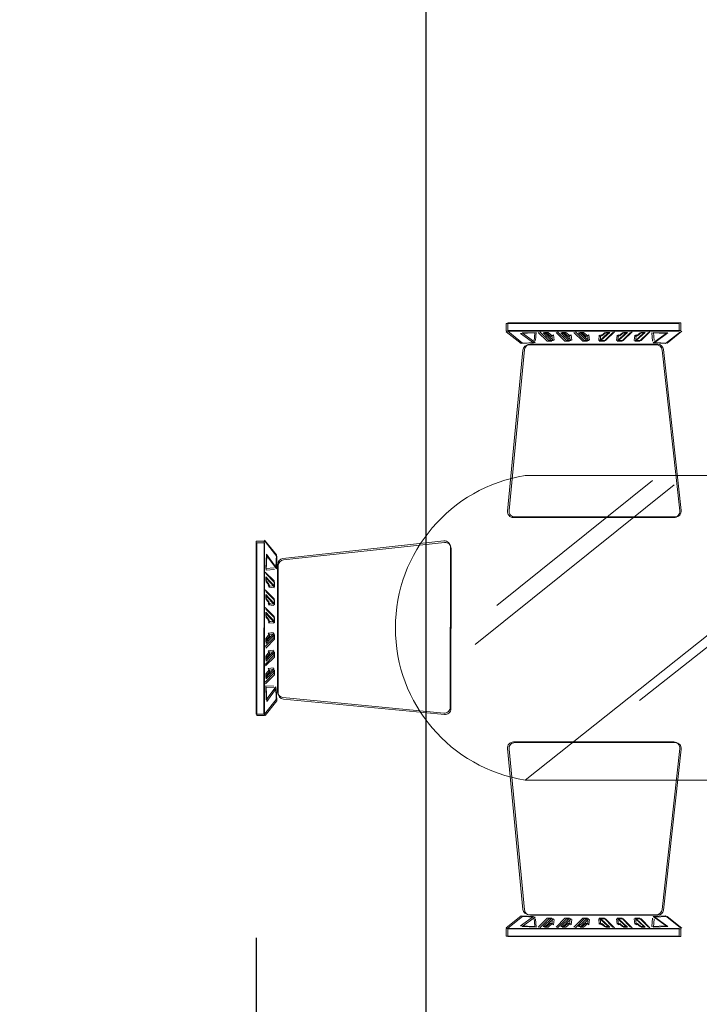
# Model space of a CAD drawing. Units: inches. Extents: x -26 to 575, y -18 to 513.
# Tile 6 of 28: x 31 to 77, y 257 to 324. Entities that reach past the tile are written whole.
import ezdxf

# ---------------------------------------------------------------- set-up
doc = ezdxf.new("R2010")
doc.units = ezdxf.units.IN
doc.header["$MEASUREMENT"] = 0
doc.layers.add('A-ANNO-DIMS', color=2, linetype='Continuous', lineweight=18)
doc.layers.add('Furniture', color=8, linetype='Continuous', lineweight=15)
doc.styles.get("Standard").update_dxf_attribs({"font": 'arial.ttf', "height": 6})
doc.dimstyles.get("Standard").update_dxf_attribs({"dimtxt": 6, "dimasz": 0.18, "dimexe": 0.18, "dimexo": 0.0625, "dimgap": 0.09, "dimtad": 0, "dimtih": 1, "dimtoh": 1, "dimzin": 0, "dimdsep": 46, "dimlunit": 3, "dimtxsty": 'Standard', "dimcen": 0.09, "dimadec": 0, "dimazin": 0, "dimtfac": 1, "dimtofl": 0, "dimtmove": 0, "dimatfit": 3, "dimfxl": 1, "dimtolj": 1, "dimtzin": 0, "dimarcsym": 0})

# ---------------------------------------------------------------- blocks, each defined once
blk = doc.blocks.new('DINING-SET-6-SEAT')
for p, q in [((16.828, 40.76, -3.573), (16.828, 41.278, -3.573)), ((16.828, 41.278, -3.573), (28.461, 41.278, -3.573)), ((16.931, 40.798, -3.573), (16.931, 41.316, -3.573)), ((16.931, 41.316, -3.573), (28.564, 41.316, -3.573)), ((28.461, 41.278, -3.573), (28.461, 40.76, -3.573)), ((28.564, 41.316, -3.573), (28.564, 40.798, -3.573)), ((47.187, 41.329, -3.573), (35.554, 41.319, -3.573)), ((35.554, 41.319, -3.573), (35.554, 40.801, -3.573)), ((47.29, 41.291, -3.573), (35.657, 41.281, -3.573)), ((35.657, 41.281, -3.573), (35.657, 40.763, -3.573)), ((47.188, 40.811, -3.573), (47.187, 41.329, -3.573)), ((47.29, 40.774, -3.573), (47.29, 41.291, -3.573)), ((28.461, 40.76, -3.573), (16.828, 40.76, -3.573)), ((16.828, 40.72, -3.573), (17.824, 39.924, -3.573)), ((28.564, 40.798, -3.573), (16.931, 40.798, -3.573)), ((16.931, 40.758, -3.573), (17.927, 39.962, -3.573)), ((17.784, 40.601, -3.573), (18.74, 40.641, -3.573)), ((18.661, 39.964, -3.573), (17.784, 40.601, -3.573)), ((17.887, 40.639, -3.573), (18.843, 40.679, -3.573)), ((18.763, 40.002, -3.573), (17.887, 40.639, -3.573)), ((18.74, 40.641, -3.573), (18.7, 40.083, -3.573)), ((18.843, 40.679, -3.573), (18.803, 40.121, -3.573)), ((18.979, 40.681, -3.573), (19.577, 40.083, -3.573)), ((19.082, 40.718, -3.573), (19.68, 40.121, -3.573)), ((19.896, 40.083, -3.573), (19.298, 40.641, -3.573)), ((19.298, 40.641, -3.573), (19.537, 40.641, -3.573)), ((19.998, 40.121, -3.573), (19.401, 40.679, -3.573)), ((19.401, 40.679, -3.573), (19.64, 40.679, -3.573)), ((19.537, 40.641, -3.573), (19.816, 40.402, -3.573)), ((19.64, 40.679, -3.573), (19.919, 40.44, -3.573)), ((19.816, 40.402, -3.573), (19.896, 40.481, -3.573)), ((19.896, 40.481, -3.573), (19.936, 40.123, -3.573)), ((19.919, 40.44, -3.573), (19.998, 40.519, -3.573)), ((19.998, 40.519, -3.573), (20.038, 40.161, -3.573)), ((20.175, 40.681, -3.573), (20.772, 40.083, -3.573)), ((20.277, 40.718, -3.573), (20.875, 40.121, -3.573)), ((21.091, 40.083, -3.573), (20.493, 40.641, -3.573)), ((20.493, 40.641, -3.573), (20.732, 40.641, -3.573)), ((21.194, 40.121, -3.573), (20.596, 40.679, -3.573)), ((20.596, 40.679, -3.573), (20.835, 40.679, -3.573)), ((20.732, 40.641, -3.573), (21.011, 40.402, -3.573)), ((20.835, 40.679, -3.573), (21.114, 40.44, -3.573)), ((21.011, 40.402, -3.573), (21.091, 40.481, -3.573)), ((21.091, 40.481, -3.573), (21.131, 40.123, -3.573)), ((21.114, 40.44, -3.573), (21.194, 40.519, -3.573)), ((21.194, 40.519, -3.573), (21.233, 40.161, -3.573)), ((21.37, 40.681, -3.573), (21.967, 40.083, -3.573)), ((21.473, 40.718, -3.573), (22.07, 40.121, -3.573)), ((22.286, 40.083, -3.573), (21.688, 40.641, -3.573)), ((21.688, 40.641, -3.573), (21.928, 40.641, -3.573)), ((22.389, 40.121, -3.573), (21.791, 40.679, -3.573)), ((21.791, 40.679, -3.573), (22.03, 40.679, -3.573)), ((21.928, 40.641, -3.573), (22.206, 40.402, -3.573)), ((22.03, 40.679, -3.573), (22.309, 40.44, -3.573)), ((22.206, 40.402, -3.573), (22.286, 40.481, -3.573)), ((22.286, 40.481, -3.573), (22.326, 40.123, -3.573)), ((22.309, 40.44, -3.573), (22.389, 40.519, -3.573)), ((22.389, 40.519, -3.573), (22.429, 40.161, -3.573)), ((23.083, 40.481, -3.573), (23.043, 40.123, -3.573)), ((23.083, 40.083, -3.573), (23.681, 40.641, -3.573)), ((23.163, 40.402, -3.573), (23.083, 40.481, -3.573)), ((23.186, 40.519, -3.573), (23.146, 40.161, -3.573)), ((23.441, 40.641, -3.573), (23.163, 40.402, -3.573)), ((23.186, 40.121, -3.573), (23.783, 40.679, -3.573)), ((23.265, 40.44, -3.573), (23.186, 40.519, -3.573)), ((23.544, 40.679, -3.573), (23.265, 40.44, -3.573)), ((23.999, 40.681, -3.573), (23.402, 40.083, -3.573)), ((23.681, 40.641, -3.573), (23.441, 40.641, -3.573)), ((24.102, 40.718, -3.573), (23.504, 40.121, -3.573)), ((23.783, 40.679, -3.573), (23.544, 40.679, -3.573)), ((24.278, 40.481, -3.573), (24.238, 40.123, -3.573)), ((24.278, 40.083, -3.573), (24.876, 40.641, -3.573)), ((24.358, 40.402, -3.573), (24.278, 40.481, -3.573)), ((24.381, 40.519, -3.573), (24.341, 40.161, -3.573)), ((24.637, 40.641, -3.573), (24.358, 40.402, -3.573)), ((24.381, 40.121, -3.573), (24.978, 40.679, -3.573)), ((24.461, 40.44, -3.573), (24.381, 40.519, -3.573)), ((24.739, 40.679, -3.573), (24.461, 40.44, -3.573)), ((25.194, 40.681, -3.573), (24.597, 40.083, -3.573)), ((24.876, 40.641, -3.573), (24.637, 40.641, -3.573)), ((25.297, 40.718, -3.573), (24.7, 40.121, -3.573)), ((24.978, 40.679, -3.573), (24.739, 40.679, -3.573)), ((25.473, 40.481, -3.573), (25.434, 40.123, -3.573)), ((25.473, 40.083, -3.573), (26.071, 40.641, -3.573)), ((25.553, 40.402, -3.573), (25.473, 40.481, -3.573)), ((25.576, 40.519, -3.573), (25.536, 40.161, -3.573)), ((25.832, 40.641, -3.573), (25.553, 40.402, -3.573)), ((25.576, 40.121, -3.573), (26.174, 40.679, -3.573)), ((25.656, 40.44, -3.573), (25.576, 40.519, -3.573)), ((25.935, 40.679, -3.573), (25.656, 40.44, -3.573)), ((26.39, 40.681, -3.573), (25.792, 40.083, -3.573)), ((26.071, 40.641, -3.573), (25.832, 40.641, -3.573)), ((26.492, 40.718, -3.573), (25.895, 40.121, -3.573)), ((26.174, 40.679, -3.573), (25.935, 40.679, -3.573)), ((27.585, 40.601, -3.573), (26.629, 40.641, -3.573)), ((26.629, 40.641, -3.573), (26.669, 40.083, -3.573)), ((26.708, 39.964, -3.573), (27.585, 40.601, -3.573)), ((27.688, 40.639, -3.573), (26.731, 40.679, -3.573)), ((26.731, 40.679, -3.573), (26.771, 40.121, -3.573)), ((26.811, 40.002, -3.573), (27.688, 40.639, -3.573)), ((28.541, 40.72, -3.573), (27.545, 39.924, -3.573)), ((28.644, 40.758, -3.573), (27.648, 39.962, -3.573)), ((35.475, 40.761, -3.573), (36.471, 39.966, -3.573)), ((35.554, 40.801, -3.573), (47.188, 40.811, -3.573)), ((35.577, 40.723, -3.573), (36.574, 39.928, -3.573)), ((35.657, 40.763, -3.573), (47.29, 40.774, -3.573)), ((36.431, 40.643, -3.573), (37.387, 40.683, -3.573)), ((37.308, 40.006, -3.573), (36.431, 40.643, -3.573)), ((36.534, 40.605, -3.573), (37.49, 40.646, -3.573)), ((37.411, 39.968, -3.573), (36.534, 40.605, -3.573)), ((37.387, 40.683, -3.573), (37.348, 40.126, -3.573)), ((37.49, 40.646, -3.573), (37.45, 40.088, -3.573)), ((37.626, 40.723, -3.573), (38.224, 40.127, -3.573)), ((37.729, 40.686, -3.573), (38.327, 40.089, -3.573)), ((38.543, 40.127, -3.573), (37.945, 40.684, -3.573)), ((37.945, 40.684, -3.573), (38.184, 40.684, -3.573)), ((38.646, 40.089, -3.573), (38.048, 40.646, -3.573)), ((38.048, 40.646, -3.573), (38.287, 40.646, -3.573)), ((38.184, 40.684, -3.573), (38.463, 40.445, -3.573)), ((38.287, 40.646, -3.573), (38.566, 40.408, -3.573)), ((38.463, 40.445, -3.573), (38.543, 40.525, -3.573)), ((38.543, 40.525, -3.573), (38.583, 40.167, -3.573)), ((38.566, 40.408, -3.573), (38.645, 40.487, -3.573)), ((38.645, 40.487, -3.573), (38.685, 40.129, -3.573)), ((38.821, 40.724, -3.573), (39.419, 40.128, -3.573)), ((38.924, 40.687, -3.573), (39.522, 40.09, -3.573)), ((39.738, 40.128, -3.573), (39.14, 40.685, -3.573)), ((39.14, 40.685, -3.573), (39.379, 40.685, -3.573)), ((39.841, 40.09, -3.573), (39.243, 40.647, -3.573)), ((39.243, 40.647, -3.573), (39.482, 40.647, -3.573)), ((39.379, 40.685, -3.573), (39.658, 40.446, -3.573)), ((39.482, 40.647, -3.573), (39.761, 40.409, -3.573)), ((39.658, 40.446, -3.573), (39.738, 40.526, -3.573)), ((39.738, 40.526, -3.573), (39.778, 40.168, -3.573)), ((39.761, 40.409, -3.573), (39.841, 40.488, -3.573)), ((39.841, 40.488, -3.573), (39.881, 40.13, -3.573)), ((40.016, 40.725, -3.573), (40.615, 40.129, -3.573)), ((40.119, 40.688, -3.573), (40.717, 40.091, -3.573)), ((40.933, 40.129, -3.573), (40.335, 40.686, -3.573)), ((40.335, 40.686, -3.573), (40.574, 40.686, -3.573)), ((41.036, 40.091, -3.573), (40.438, 40.648, -3.573)), ((40.438, 40.648, -3.573), (40.677, 40.648, -3.573)), ((40.574, 40.686, -3.573), (40.853, 40.447, -3.573)), ((40.677, 40.648, -3.573), (40.956, 40.41, -3.573)), ((40.853, 40.447, -3.573), (40.933, 40.527, -3.573)), ((40.933, 40.527, -3.573), (40.973, 40.169, -3.573)), ((40.956, 40.41, -3.573), (41.036, 40.489, -3.573)), ((41.036, 40.489, -3.573), (41.076, 40.131, -3.573)), ((41.73, 40.528, -3.573), (41.69, 40.169, -3.573)), ((41.73, 40.13, -3.573), (42.327, 40.688, -3.573)), ((41.81, 40.448, -3.573), (41.73, 40.528, -3.573)), ((41.833, 40.49, -3.573), (41.793, 40.132, -3.573)), ((42.088, 40.687, -3.573), (41.81, 40.448, -3.573)), ((41.833, 40.092, -3.573), (42.43, 40.65, -3.573)), ((41.912, 40.41, -3.573), (41.833, 40.49, -3.573)), ((42.191, 40.65, -3.573), (41.912, 40.41, -3.573)), ((42.646, 40.728, -3.573), (42.049, 40.13, -3.573)), ((42.327, 40.688, -3.573), (42.088, 40.687, -3.573)), ((42.749, 40.69, -3.573), (42.152, 40.092, -3.573)), ((42.43, 40.65, -3.573), (42.191, 40.65, -3.573)), ((42.925, 40.529, -3.573), (42.885, 40.17, -3.573)), ((42.925, 40.131, -3.573), (43.522, 40.689, -3.573)), ((43.005, 40.449, -3.573), (42.925, 40.529, -3.573)), ((43.028, 40.491, -3.573), (42.988, 40.133, -3.573)), ((43.283, 40.688, -3.573), (43.005, 40.449, -3.573)), ((43.028, 40.093, -3.573), (43.625, 40.651, -3.573)), ((43.108, 40.412, -3.573), (43.028, 40.491, -3.573)), ((43.386, 40.651, -3.573), (43.108, 40.412, -3.573)), ((43.841, 40.729, -3.573), (43.244, 40.131, -3.573)), ((43.522, 40.689, -3.573), (43.283, 40.688, -3.573)), ((43.944, 40.691, -3.573), (43.347, 40.093, -3.573)), ((43.625, 40.651, -3.573), (43.386, 40.651, -3.573)), ((44.12, 40.53, -3.573), (44.081, 40.171, -3.573)), ((44.2, 40.45, -3.573), (44.12, 40.53, -3.573)), ((44.121, 40.132, -3.573), (44.718, 40.69, -3.573)), ((44.223, 40.492, -3.573), (44.183, 40.134, -3.573)), ((44.479, 40.69, -3.573), (44.2, 40.45, -3.573)), ((44.223, 40.094, -3.573), (44.82, 40.652, -3.573)), ((44.303, 40.413, -3.573), (44.223, 40.492, -3.573)), ((44.581, 40.652, -3.573), (44.303, 40.413, -3.573)), ((45.036, 40.73, -3.573), (44.439, 40.132, -3.573)), ((44.718, 40.69, -3.573), (44.479, 40.69, -3.573)), ((45.139, 40.692, -3.573), (44.542, 40.094, -3.573)), ((44.82, 40.652, -3.573), (44.581, 40.652, -3.573)), ((46.232, 40.651, -3.573), (45.275, 40.69, -3.573)), ((45.275, 40.69, -3.573), (45.316, 40.133, -3.573)), ((45.356, 40.013, -3.573), (46.232, 40.651, -3.573)), ((46.334, 40.613, -3.573), (45.378, 40.652, -3.573)), ((45.378, 40.652, -3.573), (45.419, 40.095, -3.573)), ((45.458, 39.976, -3.573), (46.334, 40.613, -3.573)), ((47.188, 40.772, -3.573), (46.192, 39.974, -3.573)), ((47.29, 40.734, -3.573), (46.295, 39.936, -3.573)), ((17.824, 39.924, -3.573), (18.661, 39.964, -3.573)), ((17.927, 39.962, -3.573), (18.763, 40.002, -3.573)), ((26.909, 39.844, -3.573), (18.345, 39.844, -3.573)), ((27.012, 39.882, -3.573), (18.448, 39.882, -3.573)), ((19.577, 40.083, -3.573), (19.896, 40.083, -3.573)), ((19.68, 40.121, -3.573), (19.998, 40.121, -3.573)), ((20.772, 40.083, -3.573), (21.091, 40.083, -3.573)), ((20.875, 40.121, -3.573), (21.194, 40.121, -3.573)), ((21.967, 40.083, -3.573), (22.286, 40.083, -3.573)), ((22.07, 40.121, -3.573), (22.389, 40.121, -3.573)), ((23.402, 40.083, -3.573), (23.083, 40.083, -3.573)), ((23.504, 40.121, -3.573), (23.186, 40.121, -3.573)), ((24.597, 40.083, -3.573), (24.278, 40.083, -3.573)), ((24.7, 40.121, -3.573), (24.381, 40.121, -3.573)), ((25.792, 40.083, -3.573), (25.473, 40.083, -3.573)), ((25.895, 40.121, -3.573), (25.576, 40.121, -3.573)), ((27.545, 39.924, -3.573), (26.708, 39.964, -3.573)), ((27.648, 39.962, -3.573), (26.811, 40.002, -3.573)), ((36.471, 39.966, -3.573), (37.308, 40.006, -3.573)), ((36.574, 39.928, -3.573), (37.411, 39.968, -3.573)), ((37.107, 39.887, -3.573), (45.671, 39.894, -3.573)), ((37.21, 39.849, -3.573), (45.774, 39.856, -3.573)), ((38.224, 40.127, -3.573), (38.543, 40.127, -3.573)), ((38.327, 40.089, -3.573), (38.646, 40.089, -3.573)), ((39.419, 40.128, -3.573), (39.738, 40.128, -3.573)), ((39.522, 40.09, -3.573), (39.841, 40.09, -3.573)), ((40.615, 40.129, -3.573), (40.933, 40.129, -3.573)), ((40.717, 40.091, -3.573), (41.036, 40.091, -3.573)), ((42.049, 40.13, -3.573), (41.73, 40.13, -3.573)), ((42.152, 40.092, -3.573), (41.833, 40.092, -3.573)), ((43.244, 40.131, -3.573), (42.925, 40.131, -3.573)), ((43.347, 40.093, -3.573), (43.028, 40.093, -3.573)), ((44.439, 40.132, -3.573), (44.121, 40.132, -3.573)), ((44.542, 40.094, -3.573), (44.223, 40.094, -3.573)), ((46.192, 39.974, -3.573), (45.356, 40.013, -3.573)), ((46.295, 39.936, -3.573), (45.458, 39.976, -3.573)), ((17.949, 39.484, -3.573), (16.91, 28.653, -3.573)), ((18.052, 39.522, -3.573), (17.012, 28.691, -3.573)), ((28.493, 28.659, -3.573), (27.305, 39.489, -3.573)), ((28.595, 28.696, -3.573), (27.408, 39.527, -3.573)), ((35.534, 28.7, -3.573), (36.712, 39.531, -3.573)), ((35.636, 28.662, -3.573), (36.814, 39.494, -3.573)), ((46.068, 39.534, -3.573), (47.117, 28.704, -3.573)), ((46.171, 39.496, -3.573), (47.219, 28.667, -3.573)), ((16.194, 22.294, -1.308), (26.662, 30.717, -1.308)), ((46.474, 31.041, -1.308), (18.1, 31.041, -1.308)), ((14.74, 19.68, -1.308), (28.116, 30.426, -1.308)), ((25.79, 15.904, -1.308), (43.819, 30.136, -1.308)), ((17.306, 28.217, -3.573), (28.097, 28.217, -3.573)), ((17.409, 28.255, -3.573), (28.199, 28.255, -3.573)), ((46.72, 28.268, -3.573), (35.93, 28.258, -3.573)), ((46.823, 28.23, -3.573), (36.033, 28.22, -3.573)), ((18.1, 10.54, -1.308), (39.457, 27.522, -1.308)), ((0, 14.987, -3.573), (0.01, 26.621, -3.573)), ((0.01, 26.621, -3.573), (0.528, 26.62, -3.573)), ((0.037, 14.884, -3.573), (0.048, 26.518, -3.573)), ((0.048, 26.518, -3.573), (0.565, 26.517, -3.573)), ((0.528, 26.62, -3.573), (0.517, 14.987, -3.573)), ((0.565, 26.517, -3.573), (0.555, 14.884, -3.573)), ((0.567, 26.7, -3.573), (1.363, 25.703, -3.573)), ((0.605, 26.597, -3.573), (1.401, 25.6, -3.573)), ((12.629, 26.641, -3.573), (1.797, 25.463, -3.573)), ((12.667, 26.538, -3.573), (1.835, 25.36, -3.573)), ((52.057, 26.538, -3.573), (62.889, 25.36, -3.573)), ((52.095, 26.641, -3.573), (62.926, 25.463, -3.573)), ((64.119, 26.597, -3.573), (63.323, 25.6, -3.573)), ((64.156, 26.7, -3.573), (63.361, 25.703, -3.573)), ((64.676, 26.518, -3.573), (64.159, 26.517, -3.573)), ((64.159, 26.517, -3.573), (64.169, 14.884, -3.573)), ((64.714, 26.621, -3.573), (64.196, 26.62, -3.573)), ((64.196, 26.62, -3.573), (64.207, 14.987, -3.573)), ((64.686, 14.884, -3.573), (64.676, 26.518, -3.573)), ((64.724, 14.987, -3.573), (64.714, 26.621, -3.573)), ((13.061, 15.454, -3.573), (13.071, 26.244, -3.573)), ((13.099, 15.351, -3.573), (13.108, 26.142, -3.573)), ((51.625, 15.351, -3.573), (51.615, 26.142, -3.573)), ((51.663, 15.454, -3.573), (51.653, 26.244, -3.573)), ((0.686, 25.744, -3.573), (0.645, 24.787, -3.573)), ((0.724, 25.641, -3.573), (0.683, 24.685, -3.573)), ((1.322, 24.866, -3.573), (0.686, 25.744, -3.573)), ((1.36, 24.764, -3.573), (0.724, 25.641, -3.573)), ((1.363, 25.703, -3.573), (1.322, 24.866, -3.573)), ((1.401, 25.6, -3.573), (1.36, 24.764, -3.573)), ((63.323, 25.6, -3.573), (63.364, 24.764, -3.573)), ((63.361, 25.703, -3.573), (63.401, 24.866, -3.573)), ((63.364, 24.764, -3.573), (64, 25.641, -3.573)), ((63.401, 24.866, -3.573), (64.038, 25.744, -3.573)), ((64, 25.641, -3.573), (64.041, 24.685, -3.573)), ((64.038, 25.744, -3.573), (64.078, 24.787, -3.573)), ((0.605, 24.548, -3.573), (1.202, 23.95, -3.573)), ((0.645, 24.787, -3.573), (1.203, 24.827, -3.573)), ((0.683, 24.685, -3.573), (1.241, 24.724, -3.573)), ((1.442, 25.067, -3.573), (1.435, 16.503, -3.573)), ((1.48, 24.964, -3.573), (1.472, 16.401, -3.573)), ((63.244, 24.964, -3.573), (63.252, 16.401, -3.573)), ((63.282, 25.067, -3.573), (63.289, 16.503, -3.573)), ((64.041, 24.685, -3.573), (63.483, 24.724, -3.573)), ((64.078, 24.787, -3.573), (63.521, 24.827, -3.573)), ((64.118, 24.548, -3.573), (63.522, 23.95, -3.573)), ((0.643, 24.446, -3.573), (1.24, 23.847, -3.573)), ((1.202, 23.632, -3.573), (0.645, 24.23, -3.573)), ((0.645, 24.23, -3.573), (0.645, 23.991, -3.573)), ((0.645, 23.991, -3.573), (0.883, 23.712, -3.573)), ((0.683, 24.127, -3.573), (0.682, 23.888, -3.573)), ((0.682, 23.888, -3.573), (0.921, 23.609, -3.573)), ((1.24, 23.529, -3.573), (0.683, 24.127, -3.573)), ((1.202, 23.95, -3.573), (1.202, 23.632, -3.573)), ((40.039, 15.033, -1.308), (51.38, 24.327, -1.308)), ((64.081, 24.446, -3.573), (63.484, 23.847, -3.573)), ((63.484, 23.529, -3.573), (64.041, 24.127, -3.573)), ((63.522, 23.632, -3.573), (64.079, 24.23, -3.573)), ((63.522, 23.95, -3.573), (63.522, 23.632, -3.573)), ((64.041, 23.888, -3.573), (63.803, 23.609, -3.573)), ((64.079, 23.991, -3.573), (63.84, 23.712, -3.573)), ((64.041, 24.127, -3.573), (64.041, 23.888, -3.573)), ((64.079, 24.23, -3.573), (64.079, 23.991, -3.573)), ((0.604, 23.353, -3.573), (1.201, 22.755, -3.573)), ((0.642, 23.25, -3.573), (1.239, 22.652, -3.573)), ((0.883, 23.712, -3.573), (0.804, 23.632, -3.573)), ((0.804, 23.632, -3.573), (1.162, 23.592, -3.573)), ((0.921, 23.609, -3.573), (0.841, 23.529, -3.573)), ((0.841, 23.529, -3.573), (1.2, 23.489, -3.573)), ((1.24, 23.847, -3.573), (1.24, 23.529, -3.573)), ((63.484, 23.847, -3.573), (63.484, 23.529, -3.573)), ((64.082, 23.25, -3.573), (63.485, 22.652, -3.573)), ((64.12, 23.353, -3.573), (63.523, 22.755, -3.573)), ((63.882, 23.529, -3.573), (63.524, 23.489, -3.573)), ((63.92, 23.632, -3.573), (63.562, 23.592, -3.573)), ((63.803, 23.609, -3.573), (63.882, 23.529, -3.573)), ((63.84, 23.712, -3.573), (63.92, 23.632, -3.573)), ((1.201, 22.436, -3.573), (0.644, 23.034, -3.573)), ((0.644, 23.034, -3.573), (0.644, 22.795, -3.573)), ((0.644, 22.795, -3.573), (0.882, 22.516, -3.573)), ((0.682, 22.932, -3.573), (0.681, 22.693, -3.573)), ((0.681, 22.693, -3.573), (0.92, 22.414, -3.573)), ((1.239, 22.334, -3.573), (0.682, 22.932, -3.573)), ((1.201, 22.755, -3.573), (1.201, 22.436, -3.573)), ((1.239, 22.652, -3.573), (1.239, 22.334, -3.573)), ((63.485, 22.334, -3.573), (64.042, 22.932, -3.573)), ((63.485, 22.652, -3.573), (63.485, 22.334, -3.573)), ((63.523, 22.436, -3.573), (64.08, 23.034, -3.573)), ((63.523, 22.755, -3.573), (63.523, 22.436, -3.573)), ((64.042, 22.693, -3.573), (63.804, 22.414, -3.573)), ((64.08, 22.795, -3.573), (63.842, 22.516, -3.573)), ((64.042, 22.932, -3.573), (64.042, 22.693, -3.573)), ((64.08, 23.034, -3.573), (64.08, 22.795, -3.573)), ((0.603, 22.158, -3.573), (1.2, 21.56, -3.573)), ((0.641, 22.055, -3.573), (1.238, 21.457, -3.573)), ((0.882, 22.516, -3.573), (0.803, 22.437, -3.573)), ((0.803, 22.437, -3.573), (1.161, 22.397, -3.573)), ((0.92, 22.414, -3.573), (0.84, 22.334, -3.573)), ((0.84, 22.334, -3.573), (1.199, 22.294, -3.573)), ((64.083, 22.055, -3.573), (63.486, 21.457, -3.573)), ((64.121, 22.158, -3.573), (63.524, 21.56, -3.573)), ((63.883, 22.334, -3.573), (63.525, 22.294, -3.573)), ((63.921, 22.437, -3.573), (63.563, 22.397, -3.573)), ((63.804, 22.414, -3.573), (63.883, 22.334, -3.573)), ((63.842, 22.516, -3.573), (63.921, 22.437, -3.573)), ((1.2, 21.241, -3.573), (0.643, 21.839, -3.573)), ((0.643, 21.839, -3.573), (0.643, 21.6, -3.573)), ((0.643, 21.6, -3.573), (0.881, 21.321, -3.573)), ((0.681, 21.736, -3.573), (0.68, 21.497, -3.573)), ((0.68, 21.497, -3.573), (0.919, 21.218, -3.573)), ((1.238, 21.138, -3.573), (0.681, 21.736, -3.573)), ((0.881, 21.321, -3.573), (0.802, 21.241, -3.573)), ((0.802, 21.241, -3.573), (1.16, 21.201, -3.573)), ((0.919, 21.218, -3.573), (0.839, 21.139, -3.573)), ((1.2, 21.56, -3.573), (1.2, 21.241, -3.573)), ((1.238, 21.457, -3.573), (1.238, 21.138, -3.573)), ((63.486, 21.138, -3.573), (64.043, 21.736, -3.573)), ((63.486, 21.457, -3.573), (63.486, 21.138, -3.573)), ((63.524, 21.241, -3.573), (64.081, 21.839, -3.573)), ((63.524, 21.56, -3.573), (63.524, 21.241, -3.573)), ((63.922, 21.241, -3.573), (63.564, 21.201, -3.573)), ((64.043, 21.497, -3.573), (63.805, 21.218, -3.573)), ((63.805, 21.218, -3.573), (63.884, 21.139, -3.573)), ((64.081, 21.6, -3.573), (63.843, 21.321, -3.573)), ((63.843, 21.321, -3.573), (63.922, 21.241, -3.573)), ((64.043, 21.736, -3.573), (64.043, 21.497, -3.573)), ((64.081, 21.839, -3.573), (64.081, 21.6, -3.573)), ((0.839, 21.139, -3.573), (1.198, 21.099, -3.573)), ((63.884, 21.139, -3.573), (63.526, 21.099, -3.573)), ((0.601, 19.529, -3.573), (1.199, 20.126, -3.573)), ((0.639, 19.426, -3.573), (1.237, 20.023, -3.573)), ((1.199, 20.444, -3.573), (0.641, 19.847, -3.573)), ((0.641, 20.086, -3.573), (0.88, 20.365, -3.573)), ((0.641, 19.847, -3.573), (0.641, 20.086, -3.573)), ((1.237, 20.342, -3.573), (0.679, 19.744, -3.573)), ((0.679, 19.983, -3.573), (0.918, 20.262, -3.573)), ((0.679, 19.744, -3.573), (0.679, 19.983, -3.573)), ((0.801, 20.445, -3.573), (1.159, 20.484, -3.573)), ((0.88, 20.365, -3.573), (0.801, 20.445, -3.573)), ((0.839, 20.342, -3.573), (1.197, 20.381, -3.573)), ((0.918, 20.262, -3.573), (0.839, 20.342, -3.573)), ((1.199, 20.126, -3.573), (1.199, 20.444, -3.573)), ((1.237, 20.023, -3.573), (1.237, 20.342, -3.573)), ((34.805, 10.386, -1.308), (47.018, 19.971, -1.308)), ((63.487, 20.023, -3.573), (63.487, 20.342, -3.573)), ((63.487, 20.342, -3.573), (64.045, 19.744, -3.573)), ((64.085, 19.426, -3.573), (63.487, 20.023, -3.573)), ((63.525, 20.126, -3.573), (63.525, 20.444, -3.573)), ((63.525, 20.444, -3.573), (64.083, 19.847, -3.573)), ((64.123, 19.529, -3.573), (63.525, 20.126, -3.573)), ((63.885, 20.342, -3.573), (63.527, 20.381, -3.573)), ((63.923, 20.445, -3.573), (63.565, 20.484, -3.573)), ((63.806, 20.262, -3.573), (63.885, 20.342, -3.573)), ((64.045, 19.983, -3.573), (63.806, 20.262, -3.573)), ((63.843, 20.365, -3.573), (63.923, 20.445, -3.573)), ((64.083, 20.086, -3.573), (63.843, 20.365, -3.573)), ((64.045, 19.744, -3.573), (64.045, 19.983, -3.573)), ((64.083, 19.847, -3.573), (64.083, 20.086, -3.573)), ((1.198, 19.249, -3.573), (0.64, 18.652, -3.573)), ((0.8, 19.249, -3.573), (1.158, 19.289, -3.573)), ((0.879, 19.17, -3.573), (0.8, 19.249, -3.573)), ((1.198, 18.93, -3.573), (1.198, 19.249, -3.573)), ((63.526, 18.93, -3.573), (63.526, 19.249, -3.573)), ((63.526, 19.249, -3.573), (64.084, 18.652, -3.573)), ((63.924, 19.249, -3.573), (63.566, 19.289, -3.573)), ((63.844, 19.17, -3.573), (63.924, 19.249, -3.573)), ((0.6, 18.333, -3.573), (1.198, 18.93, -3.573)), ((0.638, 18.231, -3.573), (1.236, 18.828, -3.573)), ((0.64, 18.891, -3.573), (0.879, 19.17, -3.573)), ((0.64, 18.652, -3.573), (0.64, 18.891, -3.573)), ((1.236, 19.146, -3.573), (0.678, 18.549, -3.573)), ((0.678, 18.788, -3.573), (0.917, 19.067, -3.573)), ((0.678, 18.549, -3.573), (0.678, 18.788, -3.573)), ((0.838, 19.147, -3.573), (1.196, 19.186, -3.573)), ((0.917, 19.067, -3.573), (0.838, 19.147, -3.573)), ((1.236, 18.828, -3.573), (1.236, 19.146, -3.573)), ((63.488, 18.828, -3.573), (63.488, 19.146, -3.573)), ((63.488, 19.146, -3.573), (64.046, 18.549, -3.573)), ((64.086, 18.231, -3.573), (63.488, 18.828, -3.573)), ((64.124, 18.333, -3.573), (63.526, 18.93, -3.573)), ((63.886, 19.147, -3.573), (63.528, 19.186, -3.573)), ((63.807, 19.067, -3.573), (63.886, 19.147, -3.573)), ((64.046, 18.788, -3.573), (63.807, 19.067, -3.573)), ((64.084, 18.891, -3.573), (63.844, 19.17, -3.573)), ((64.046, 18.549, -3.573), (64.046, 18.788, -3.573)), ((64.084, 18.652, -3.573), (64.084, 18.891, -3.573)), ((1.197, 18.054, -3.573), (0.639, 17.457, -3.573)), ((0.639, 17.696, -3.573), (0.878, 17.974, -3.573)), ((1.235, 17.951, -3.573), (0.677, 17.354, -3.573)), ((0.799, 18.054, -3.573), (1.157, 18.094, -3.573)), ((0.878, 17.974, -3.573), (0.799, 18.054, -3.573)), ((0.837, 17.951, -3.573), (1.195, 17.991, -3.573)), ((0.916, 17.872, -3.573), (0.837, 17.951, -3.573)), ((1.197, 17.735, -3.573), (1.197, 18.054, -3.573)), ((1.234, 17.632, -3.573), (1.235, 17.951, -3.573)), ((63.489, 17.632, -3.573), (63.489, 17.951, -3.573)), ((63.489, 17.951, -3.573), (64.047, 17.354, -3.573)), ((63.527, 17.735, -3.573), (63.527, 18.054, -3.573)), ((63.527, 18.054, -3.573), (64.085, 17.457, -3.573)), ((63.887, 17.951, -3.573), (63.529, 17.991, -3.573)), ((63.925, 18.054, -3.573), (63.567, 18.094, -3.573)), ((63.808, 17.872, -3.573), (63.887, 17.951, -3.573)), ((63.846, 17.974, -3.573), (63.925, 18.054, -3.573)), ((64.085, 17.696, -3.573), (63.846, 17.974, -3.573)), ((0.599, 17.138, -3.573), (1.197, 17.735, -3.573)), ((0.637, 17.035, -3.573), (1.234, 17.632, -3.573)), ((0.639, 17.457, -3.573), (0.639, 17.696, -3.573)), ((0.677, 17.593, -3.573), (0.916, 17.872, -3.573)), ((0.677, 17.354, -3.573), (0.677, 17.593, -3.573)), ((64.087, 17.035, -3.573), (63.489, 17.632, -3.573)), ((64.125, 17.138, -3.573), (63.527, 17.735, -3.573)), ((64.047, 17.593, -3.573), (63.808, 17.872, -3.573)), ((64.047, 17.354, -3.573), (64.047, 17.593, -3.573)), ((64.085, 17.457, -3.573), (64.085, 17.696, -3.573)), ((0.677, 15.943, -3.573), (0.639, 16.899, -3.573)), ((0.639, 16.899, -3.573), (1.196, 16.859, -3.573)), ((0.715, 15.84, -3.573), (0.676, 16.796, -3.573)), ((0.676, 16.796, -3.573), (1.234, 16.756, -3.573)), ((1.315, 16.819, -3.573), (0.677, 15.943, -3.573)), ((1.353, 16.716, -3.573), (0.715, 15.84, -3.573)), ((1.354, 15.982, -3.573), (1.315, 16.819, -3.573)), ((1.392, 15.879, -3.573), (1.353, 16.716, -3.573)), ((63.332, 15.879, -3.573), (63.371, 16.716, -3.573)), ((63.369, 15.982, -3.573), (63.408, 16.819, -3.573)), ((63.371, 16.716, -3.573), (64.009, 15.84, -3.573)), ((63.408, 16.819, -3.573), (64.046, 15.943, -3.573)), ((64.048, 16.796, -3.573), (63.49, 16.756, -3.573)), ((64.085, 16.899, -3.573), (63.528, 16.859, -3.573)), ((64.009, 15.84, -3.573), (64.048, 16.796, -3.573)), ((64.046, 15.943, -3.573), (64.085, 16.899, -3.573)), ((0.557, 14.987, -3.573), (1.354, 15.982, -3.573)), ((1.795, 16.106, -3.573), (12.624, 15.058, -3.573)), ((1.832, 16.004, -3.573), (12.662, 14.955, -3.573)), ((62.892, 16.004, -3.573), (52.062, 14.955, -3.573)), ((62.929, 16.106, -3.573), (52.099, 15.058, -3.573)), ((64.167, 14.987, -3.573), (63.369, 15.982, -3.573)), ((0.595, 14.884, -3.573), (1.392, 15.879, -3.573)), ((64.129, 14.884, -3.573), (63.332, 15.879, -3.573)), ((0.517, 14.987, -3.573), (0, 14.987, -3.573)), ((0.555, 14.884, -3.573), (0.037, 14.884, -3.573)), ((64.169, 14.884, -3.573), (64.686, 14.884, -3.573)), ((64.207, 14.987, -3.573), (64.724, 14.987, -3.573)), ((17.949, 1.845, -3.573), (16.91, 12.676, -3.573)), ((18.052, 1.807, -3.573), (17.012, 12.638, -3.573)), ((17.306, 13.113, -3.573), (28.097, 13.113, -3.573)), ((17.409, 13.075, -3.573), (28.199, 13.075, -3.573)), ((28.493, 12.671, -3.573), (27.305, 1.84, -3.573)), ((28.595, 12.633, -3.573), (27.408, 1.802, -3.573)), ((35.534, 12.63, -3.573), (36.712, 1.798, -3.573)), ((35.636, 12.668, -3.573), (36.814, 1.836, -3.573)), ((46.72, 13.062, -3.573), (35.93, 13.071, -3.573)), ((46.823, 13.1, -3.573), (36.033, 13.109, -3.573)), ((46.068, 1.795, -3.573), (47.117, 12.625, -3.573)), ((46.171, 1.833, -3.573), (47.219, 12.663, -3.573)), ((18.1, 10.54, -1.308), (46.474, 10.54, -1.308)), ((16.828, 0.609, -3.573), (17.824, 1.405, -3.573)), ((16.931, 0.571, -3.573), (17.927, 1.367, -3.573)), ((18.661, 1.366, -3.573), (17.784, 0.728, -3.573)), ((17.824, 1.405, -3.573), (18.661, 1.366, -3.573)), ((18.763, 1.328, -3.573), (17.887, 0.691, -3.573)), ((17.927, 1.367, -3.573), (18.763, 1.328, -3.573)), ((26.909, 1.485, -3.573), (18.345, 1.485, -3.573)), ((27.012, 1.447, -3.573), (18.448, 1.447, -3.573)), ((27.545, 1.405, -3.573), (26.708, 1.366, -3.573)), ((26.708, 1.366, -3.573), (27.585, 0.728, -3.573)), ((27.648, 1.367, -3.573), (26.811, 1.328, -3.573)), ((26.811, 1.328, -3.573), (27.688, 0.691, -3.573)), ((28.541, 0.609, -3.573), (27.545, 1.405, -3.573)), ((28.644, 0.571, -3.573), (27.648, 1.367, -3.573)), ((35.475, 0.568, -3.573), (36.471, 1.364, -3.573)), ((35.577, 0.606, -3.573), (36.574, 1.401, -3.573)), ((36.471, 1.364, -3.573), (37.308, 1.323, -3.573)), ((37.411, 1.361, -3.573), (36.534, 0.724, -3.573)), ((36.574, 1.401, -3.573), (37.411, 1.361, -3.573)), ((37.107, 1.443, -3.573), (45.671, 1.435, -3.573)), ((37.21, 1.48, -3.573), (45.774, 1.473, -3.573)), ((46.192, 1.355, -3.573), (45.356, 1.316, -3.573)), ((46.295, 1.393, -3.573), (45.458, 1.354, -3.573)), ((45.458, 1.354, -3.573), (46.334, 0.716, -3.573)), ((47.188, 0.558, -3.573), (46.192, 1.355, -3.573)), ((47.29, 0.596, -3.573), (46.295, 1.393, -3.573)), ((17.784, 0.728, -3.573), (18.74, 0.689, -3.573)), ((17.887, 0.691, -3.573), (18.843, 0.651, -3.573)), ((18.74, 0.689, -3.573), (18.7, 1.246, -3.573)), ((18.843, 0.651, -3.573), (18.803, 1.208, -3.573)), ((18.979, 0.649, -3.573), (19.577, 1.246, -3.573)), ((19.082, 0.611, -3.573), (19.68, 1.208, -3.573)), ((19.896, 1.246, -3.573), (19.298, 0.689, -3.573)), ((19.298, 0.689, -3.573), (19.537, 0.689, -3.573)), ((19.998, 1.208, -3.573), (19.401, 0.651, -3.573)), ((19.537, 0.689, -3.573), (19.816, 0.928, -3.573)), ((19.577, 1.246, -3.573), (19.896, 1.246, -3.573)), ((19.64, 0.651, -3.573), (19.919, 0.89, -3.573)), ((19.68, 1.208, -3.573), (19.998, 1.208, -3.573)), ((19.816, 0.928, -3.573), (19.896, 0.848, -3.573)), ((19.896, 0.848, -3.573), (19.936, 1.206, -3.573)), ((19.919, 0.89, -3.573), (19.998, 0.81, -3.573)), ((19.998, 0.81, -3.573), (20.038, 1.168, -3.573)), ((20.175, 0.649, -3.573), (20.772, 1.246, -3.573)), ((20.277, 0.611, -3.573), (20.875, 1.208, -3.573)), ((21.091, 1.246, -3.573), (20.493, 0.689, -3.573)), ((20.493, 0.689, -3.573), (20.732, 0.689, -3.573)), ((21.194, 1.208, -3.573), (20.596, 0.651, -3.573)), ((20.732, 0.689, -3.573), (21.011, 0.928, -3.573)), ((20.772, 1.246, -3.573), (21.091, 1.246, -3.573)), ((20.835, 0.651, -3.573), (21.114, 0.89, -3.573)), ((20.875, 1.208, -3.573), (21.194, 1.208, -3.573)), ((21.011, 0.928, -3.573), (21.091, 0.848, -3.573)), ((21.091, 0.848, -3.573), (21.131, 1.206, -3.573)), ((21.114, 0.89, -3.573), (21.194, 0.81, -3.573)), ((21.194, 0.81, -3.573), (21.233, 1.168, -3.573)), ((21.37, 0.649, -3.573), (21.967, 1.246, -3.573)), ((21.473, 0.611, -3.573), (22.07, 1.208, -3.573)), ((22.286, 1.246, -3.573), (21.688, 0.689, -3.573)), ((21.688, 0.689, -3.573), (21.928, 0.689, -3.573)), ((22.389, 1.208, -3.573), (21.791, 0.651, -3.573)), ((21.928, 0.689, -3.573), (22.206, 0.928, -3.573)), ((21.967, 1.246, -3.573), (22.286, 1.246, -3.573)), ((22.03, 0.651, -3.573), (22.309, 0.89, -3.573)), ((22.07, 1.208, -3.573), (22.389, 1.208, -3.573)), ((22.206, 0.928, -3.573), (22.286, 0.848, -3.573)), ((22.286, 0.848, -3.573), (22.326, 1.206, -3.573)), ((22.309, 0.89, -3.573), (22.389, 0.81, -3.573)), ((22.389, 0.81, -3.573), (22.429, 1.168, -3.573)), ((23.083, 0.848, -3.573), (23.043, 1.206, -3.573)), ((23.402, 1.246, -3.573), (23.083, 1.246, -3.573)), ((23.083, 1.246, -3.573), (23.681, 0.689, -3.573)), ((23.163, 0.928, -3.573), (23.083, 0.848, -3.573)), ((23.186, 0.81, -3.573), (23.146, 1.168, -3.573)), ((23.441, 0.689, -3.573), (23.163, 0.928, -3.573)), ((23.504, 1.208, -3.573), (23.186, 1.208, -3.573)), ((23.186, 1.208, -3.573), (23.783, 0.651, -3.573)), ((23.265, 0.89, -3.573), (23.186, 0.81, -3.573)), ((23.544, 0.651, -3.573), (23.265, 0.89, -3.573)), ((23.999, 0.649, -3.573), (23.402, 1.246, -3.573)), ((23.681, 0.689, -3.573), (23.441, 0.689, -3.573)), ((24.102, 0.611, -3.573), (23.504, 1.208, -3.573)), ((24.278, 0.848, -3.573), (24.238, 1.206, -3.573)), ((24.597, 1.246, -3.573), (24.278, 1.246, -3.573)), ((24.278, 1.246, -3.573), (24.876, 0.689, -3.573)), ((24.358, 0.928, -3.573), (24.278, 0.848, -3.573)), ((24.381, 0.81, -3.573), (24.341, 1.168, -3.573)), ((24.637, 0.689, -3.573), (24.358, 0.928, -3.573)), ((24.7, 1.208, -3.573), (24.381, 1.208, -3.573)), ((24.381, 1.208, -3.573), (24.978, 0.651, -3.573)), ((24.461, 0.89, -3.573), (24.381, 0.81, -3.573)), ((24.739, 0.651, -3.573), (24.461, 0.89, -3.573)), ((25.194, 0.649, -3.573), (24.597, 1.246, -3.573)), ((24.876, 0.689, -3.573), (24.637, 0.689, -3.573)), ((25.297, 0.611, -3.573), (24.7, 1.208, -3.573)), ((25.473, 0.848, -3.573), (25.434, 1.206, -3.573)), ((25.792, 1.246, -3.573), (25.473, 1.246, -3.573)), ((25.473, 1.246, -3.573), (26.071, 0.689, -3.573)), ((25.553, 0.928, -3.573), (25.473, 0.848, -3.573)), ((25.576, 0.81, -3.573), (25.536, 1.168, -3.573)), ((25.832, 0.689, -3.573), (25.553, 0.928, -3.573)), ((25.895, 1.208, -3.573), (25.576, 1.208, -3.573)), ((25.576, 1.208, -3.573), (26.174, 0.651, -3.573)), ((25.656, 0.89, -3.573), (25.576, 0.81, -3.573)), ((25.935, 0.651, -3.573), (25.656, 0.89, -3.573)), ((26.39, 0.649, -3.573), (25.792, 1.246, -3.573)), ((26.071, 0.689, -3.573), (25.832, 0.689, -3.573)), ((26.492, 0.611, -3.573), (25.895, 1.208, -3.573)), ((26.629, 0.689, -3.573), (26.669, 1.246, -3.573)), ((27.585, 0.728, -3.573), (26.629, 0.689, -3.573)), ((26.731, 0.651, -3.573), (26.771, 1.208, -3.573)), ((27.688, 0.691, -3.573), (26.731, 0.651, -3.573)), ((37.308, 1.323, -3.573), (36.431, 0.687, -3.573)), ((36.431, 0.687, -3.573), (37.387, 0.646, -3.573)), ((36.534, 0.724, -3.573), (37.49, 0.684, -3.573)), ((37.387, 0.646, -3.573), (37.348, 1.204, -3.573)), ((37.49, 0.684, -3.573), (37.45, 1.241, -3.573)), ((37.626, 0.606, -3.573), (38.224, 1.203, -3.573)), ((37.729, 0.644, -3.573), (38.327, 1.241, -3.573)), ((38.543, 1.203, -3.573), (37.945, 0.646, -3.573)), ((38.646, 1.24, -3.573), (38.048, 0.683, -3.573)), ((38.048, 0.683, -3.573), (38.287, 0.683, -3.573)), ((38.184, 0.645, -3.573), (38.463, 0.884, -3.573)), ((38.224, 1.203, -3.573), (38.543, 1.203, -3.573)), ((38.287, 0.683, -3.573), (38.566, 0.922, -3.573)), ((38.327, 1.241, -3.573), (38.646, 1.24, -3.573)), ((38.463, 0.884, -3.573), (38.543, 0.804, -3.573)), ((38.543, 0.804, -3.573), (38.583, 1.163, -3.573)), ((38.566, 0.922, -3.573), (38.645, 0.842, -3.573)), ((38.645, 0.842, -3.573), (38.685, 1.2, -3.573)), ((38.821, 0.605, -3.573), (39.419, 1.202, -3.573)), ((38.924, 0.643, -3.573), (39.522, 1.24, -3.573)), ((39.738, 1.201, -3.573), (39.14, 0.645, -3.573)), ((39.841, 1.239, -3.573), (39.243, 0.682, -3.573)), ((39.243, 0.682, -3.573), (39.482, 0.682, -3.573)), ((39.379, 0.644, -3.573), (39.658, 0.883, -3.573)), ((39.419, 1.202, -3.573), (39.738, 1.201, -3.573)), ((39.482, 0.682, -3.573), (39.761, 0.921, -3.573)), ((39.522, 1.24, -3.573), (39.841, 1.239, -3.573)), ((39.658, 0.883, -3.573), (39.738, 0.803, -3.573)), ((39.738, 0.803, -3.573), (39.778, 1.162, -3.573)), ((39.761, 0.921, -3.573), (39.841, 0.841, -3.573)), ((39.841, 0.841, -3.573), (39.881, 1.199, -3.573)), ((40.016, 0.604, -3.573), (40.615, 1.201, -3.573)), ((40.119, 0.642, -3.573), (40.717, 1.238, -3.573)), ((40.933, 1.2, -3.573), (40.335, 0.643, -3.573)), ((41.036, 1.238, -3.573), (40.438, 0.681, -3.573)), ((40.438, 0.681, -3.573), (40.677, 0.681, -3.573)), ((40.574, 0.643, -3.573), (40.853, 0.882, -3.573)), ((40.615, 1.201, -3.573), (40.933, 1.2, -3.573)), ((40.677, 0.681, -3.573), (40.956, 0.92, -3.573)), ((40.717, 1.238, -3.573), (41.036, 1.238, -3.573)), ((40.853, 0.882, -3.573), (40.933, 0.802, -3.573)), ((40.933, 0.802, -3.573), (40.973, 1.161, -3.573)), ((40.956, 0.92, -3.573), (41.036, 0.84, -3.573)), ((41.036, 0.84, -3.573), (41.076, 1.198, -3.573)), ((41.73, 0.802, -3.573), (41.69, 1.16, -3.573)), ((42.049, 1.199, -3.573), (41.73, 1.2, -3.573)), ((41.73, 1.2, -3.573), (42.327, 0.642, -3.573)), ((41.81, 0.881, -3.573), (41.73, 0.802, -3.573)), ((41.833, 0.839, -3.573), (41.793, 1.198, -3.573)), ((42.088, 0.642, -3.573), (41.81, 0.881, -3.573)), ((42.152, 1.237, -3.573), (41.833, 1.238, -3.573)), ((41.833, 1.238, -3.573), (42.43, 0.679, -3.573)), ((41.912, 0.919, -3.573), (41.833, 0.839, -3.573)), ((42.191, 0.68, -3.573), (41.912, 0.919, -3.573)), ((42.646, 0.602, -3.573), (42.049, 1.199, -3.573)), ((42.749, 0.639, -3.573), (42.152, 1.237, -3.573)), ((42.43, 0.679, -3.573), (42.191, 0.68, -3.573)), ((42.925, 0.8, -3.573), (42.885, 1.159, -3.573)), ((43.244, 1.198, -3.573), (42.925, 1.199, -3.573)), ((42.925, 1.199, -3.573), (43.522, 0.641, -3.573)), ((43.005, 0.88, -3.573), (42.925, 0.8, -3.573)), ((43.028, 0.838, -3.573), (42.988, 1.197, -3.573)), ((43.283, 0.641, -3.573), (43.005, 0.88, -3.573)), ((43.347, 1.236, -3.573), (43.028, 1.236, -3.573)), ((43.028, 1.236, -3.573), (43.625, 0.678, -3.573)), ((43.108, 0.918, -3.573), (43.028, 0.838, -3.573)), ((43.386, 0.679, -3.573), (43.108, 0.918, -3.573)), ((43.841, 0.601, -3.573), (43.244, 1.198, -3.573)), ((43.944, 0.638, -3.573), (43.347, 1.236, -3.573)), ((43.625, 0.678, -3.573), (43.386, 0.679, -3.573)), ((44.12, 0.799, -3.573), (44.081, 1.158, -3.573)), ((44.2, 0.879, -3.573), (44.12, 0.799, -3.573)), ((44.439, 1.197, -3.573), (44.121, 1.198, -3.573)), ((44.121, 1.198, -3.573), (44.718, 0.64, -3.573)), ((44.223, 0.837, -3.573), (44.183, 1.196, -3.573)), ((44.479, 0.64, -3.573), (44.2, 0.879, -3.573)), ((44.542, 1.235, -3.573), (44.223, 1.235, -3.573)), ((44.223, 1.235, -3.573), (44.82, 0.677, -3.573)), ((44.303, 0.917, -3.573), (44.223, 0.837, -3.573)), ((44.581, 0.678, -3.573), (44.303, 0.917, -3.573)), ((45.036, 0.6, -3.573), (44.439, 1.197, -3.573)), ((45.139, 0.637, -3.573), (44.542, 1.235, -3.573)), ((44.82, 0.677, -3.573), (44.581, 0.678, -3.573)), ((45.275, 0.639, -3.573), (45.316, 1.197, -3.573)), ((46.232, 0.678, -3.573), (45.275, 0.639, -3.573)), ((45.356, 1.316, -3.573), (46.232, 0.678, -3.573)), ((45.378, 0.677, -3.573), (45.419, 1.234, -3.573)), ((46.334, 0.716, -3.573), (45.378, 0.677, -3.573)), ((28.461, 0.569, -3.573), (16.828, 0.569, -3.573)), ((16.828, 0.569, -3.573), (16.828, 0.051, -3.573)), ((16.828, 0.051, -3.573), (28.461, 0.051, -3.573)), ((28.564, 0.531, -3.573), (16.931, 0.531, -3.573)), ((16.931, 0.531, -3.573), (16.931, 0.014, -3.573)), ((16.931, 0.014, -3.573), (28.564, 0.014, -3.573)), ((19.401, 0.651, -3.573), (19.64, 0.651, -3.573)), ((20.596, 0.651, -3.573), (20.835, 0.651, -3.573)), ((21.791, 0.651, -3.573), (22.03, 0.651, -3.573)), ((23.783, 0.651, -3.573), (23.544, 0.651, -3.573)), ((24.978, 0.651, -3.573), (24.739, 0.651, -3.573)), ((26.174, 0.651, -3.573), (25.935, 0.651, -3.573)), ((28.461, 0.051, -3.573), (28.461, 0.569, -3.573)), ((28.564, 0.014, -3.573), (28.564, 0.531, -3.573)), ((35.554, 0.011, -3.573), (35.554, 0.528, -3.573)), ((35.554, 0.528, -3.573), (47.188, 0.518, -3.573)), ((47.187, 0, -3.573), (35.554, 0.011, -3.573)), ((35.657, 0.048, -3.573), (35.657, 0.566, -3.573)), ((35.657, 0.566, -3.573), (47.29, 0.556, -3.573)), ((47.29, 0.038, -3.573), (35.657, 0.048, -3.573)), ((37.945, 0.646, -3.573), (38.184, 0.645, -3.573)), ((39.14, 0.645, -3.573), (39.379, 0.644, -3.573)), ((40.335, 0.643, -3.573), (40.574, 0.643, -3.573)), ((42.327, 0.642, -3.573), (42.088, 0.642, -3.573)), ((43.522, 0.641, -3.573), (43.283, 0.641, -3.573)), ((44.718, 0.64, -3.573), (44.479, 0.64, -3.573)), ((47.188, 0.518, -3.573), (47.187, 0, -3.573)), ((47.29, 0.556, -3.573), (47.29, 0.038, -3.573))]:
    blk.add_line(p, q)
for centre, radius, start, end in [((18.345, 39.446, -3.573), 0.398, 90, 174.51988), ((18.448, 39.484, -3.573), 0.398, 90, 174.51988), ((26.909, 39.446, -3.573), 0.398, 6.25717, 90), ((27.012, 39.484, -3.573), 0.398, 6.25717, 90), ((37.108, 39.488, -3.573), 0.398, 90.05022, 173.79305), ((37.211, 39.45, -3.573), 0.398, 90.05022, 173.79305), ((45.671, 39.496, -3.573), 0.398, 5.53034, 90.05022), ((45.774, 39.458, -3.573), 0.398, 5.53034, 90.05022), ((19.748, 20.791, -1.308), 10.382, 99.13208, 260.86792), ((44.826, 20.791, -1.308), 10.382, 279.13208, 80.86792), ((17.306, 28.615, -3.573), 0.398, 174.51988, 270), ((17.409, 28.653, -3.573), 0.398, 174.51988, 270), ((28.097, 28.615, -3.573), 0.398, 270, 6.25717), ((28.199, 28.653, -3.573), 0.398, 270, 6.25717), ((35.93, 28.656, -3.573), 0.398, 173.79305, 270.05022), ((36.032, 28.619, -3.573), 0.398, 173.79305, 270.05022), ((46.72, 28.666, -3.573), 0.398, 270.05022, 5.53034), ((46.823, 28.628, -3.573), 0.398, 270.05022, 5.53034), ((12.672, 26.245, -3.573), 0.398, 359.94978, 96.20695), ((12.71, 26.142, -3.573), 0.398, 359.94978, 96.20695), ((52.014, 26.142, -3.573), 0.398, 83.79305, 180.05022), ((52.052, 26.245, -3.573), 0.398, 83.79305, 180.05022), ((1.84, 25.067, -3.573), 0.398, 96.20695, 179.94978), ((1.878, 24.964, -3.573), 0.398, 96.20695, 179.94978), ((62.846, 24.964, -3.573), 0.398, 0.05022, 83.79305), ((62.883, 25.067, -3.573), 0.398, 0.05022, 83.79305), ((1.833, 16.503, -3.573), 0.398, 179.94978, 264.46966), ((1.871, 16.4, -3.573), 0.398, 179.94978, 264.46966), ((62.853, 16.4, -3.573), 0.398, 275.53034, 0.05022), ((62.891, 16.503, -3.573), 0.398, 275.53034, 0.05022), ((12.663, 15.454, -3.573), 0.398, 264.46966, 359.94978), ((12.701, 15.352, -3.573), 0.398, 264.46966, 359.94978), ((52.023, 15.352, -3.573), 0.398, 180.05022, 275.53034), ((52.061, 15.454, -3.573), 0.398, 180.05022, 275.53034), ((17.306, 12.714, -3.573), 0.398, 90, 185.48012), ((17.409, 12.676, -3.573), 0.398, 90, 185.48012), ((28.097, 12.714, -3.573), 0.398, 353.74283, 90), ((28.199, 12.676, -3.573), 0.398, 353.74283, 90), ((35.93, 12.673, -3.573), 0.398, 89.94978, 186.20695), ((36.032, 12.711, -3.573), 0.398, 89.94978, 186.20695), ((46.72, 12.663, -3.573), 0.398, 354.46966, 89.94978), ((46.823, 12.701, -3.573), 0.398, 354.46966, 89.94978), ((18.345, 1.883, -3.573), 0.398, 185.48012, 270), ((18.448, 1.846, -3.573), 0.398, 185.48012, 270), ((26.909, 1.883, -3.573), 0.398, 270, 353.74283), ((27.012, 1.846, -3.573), 0.398, 270, 353.74283), ((37.108, 1.841, -3.573), 0.398, 186.20695, 269.94978), ((37.211, 1.879, -3.573), 0.398, 186.20695, 269.94978), ((45.671, 1.834, -3.573), 0.398, 269.94978, 354.46966), ((45.774, 1.871, -3.573), 0.398, 269.94978, 354.46966)]:
    blk.add_arc(centre, radius, start, end)
blk = doc.blocks.new('*D24')
at = {"layer": 'A-ANNO-DIMS', "color": 0, "lineweight": -2, "transparency": 16777216}
for p, q in [((46.82, 261.725), (46.82, 251.899)), ((111.544, 261.725), (111.544, 251.899)), ((47, 252.079), (111.364, 252.079)), ((111.544, 252.079), (111.724, 252.079))]:
    blk.add_line(p, q, dxfattribs=at)
at = {"layer": 'A-ANNO-DIMS', "color": 0, "transparency": 16777216}
for points in [[(47, 252.109), (47, 252.049), (46.82, 252.079)], [(111.364, 252.109), (111.364, 252.049), (111.544, 252.079)]]:
    blk.add_solid(points, dxfattribs=at)
at = {"layer": 'Defpoints', "color": 0, "transparency": 16777216}
for p in [(46.82, 261.787), (111.544, 261.787), (111.544, 252.079)]:
    blk.add_point(p, dxfattribs=at)
at = {"layer": 'A-ANNO-DIMS', "color": 0, "transparency": 16777216, "insert": (162.09, 252.079), "char_height": 6, "attachment_point": 5}
blk.add_mtext('\\A1;DINING SET 5\'-4 1/2" TYP.', dxfattribs=at)
blk = doc.blocks.new('*D28')
at = {"layer": 'A-ANNO-DIMS', "color": 0, "lineweight": -2, "transparency": 16777216}
for p, q in [((58.224, 466.445), (58.224, -8.972)), ((95.349, 466.445), (95.349, -8.972)), ((58.404, -8.792), (68.723, -8.792)), ((95.169, -8.792), (84.849, -8.792))]:
    blk.add_line(p, q, dxfattribs=at)
at = {"layer": 'A-ANNO-DIMS', "color": 0, "transparency": 16777216}
for points in [[(58.404, -8.762), (58.404, -8.822), (58.224, -8.792)], [(95.169, -8.762), (95.169, -8.822), (95.349, -8.792)]]:
    blk.add_solid(points, dxfattribs=at)
at = {"layer": 'Defpoints', "color": 0, "transparency": 16777216}
for p in [(58.224, 466.508), (95.349, 466.508), (95.349, -8.792)]:
    blk.add_point(p, dxfattribs=at)
at = {"layer": 'A-ANNO-DIMS', "color": 0, "transparency": 16777216, "insert": (76.786, -8.792), "char_height": 6, "attachment_point": 5}
blk.add_mtext('\\A1;3\'-1"', dxfattribs=at)
blk = doc.blocks.new('*D50')
at = {"layer": 'A-ANNO-DIMS', "color": 0, "lineweight": -2, "transparency": 16777216}
for p, q in [((27.177, 466.445), (27.177, -8.972)), ((58.224, 466.445), (58.224, -8.972)), ((27.357, -8.792), (34.584, -8.792)), ((58.044, -8.792), (50.816, -8.792))]:
    blk.add_line(p, q, dxfattribs=at)
at = {"layer": 'A-ANNO-DIMS', "color": 0, "transparency": 16777216}
for points in [[(27.357, -8.762), (27.357, -8.822), (27.177, -8.792)], [(58.044, -8.762), (58.044, -8.822), (58.224, -8.792)]]:
    blk.add_solid(points, dxfattribs=at)
at = {"layer": 'Defpoints', "color": 0, "transparency": 16777216}
for p in [(27.177, 466.508), (58.224, 466.508), (58.224, -8.792)]:
    blk.add_point(p, dxfattribs=at)
at = {"layer": 'A-ANNO-DIMS', "color": 0, "transparency": 16777216, "insert": (42.7, -8.792), "char_height": 6, "attachment_point": 5}
blk.add_mtext('\\A1;2\'-7"', dxfattribs=at)

msp = doc.modelspace()

# ---------------------------------------------------------------- block references
at = {"layer": 'Furniture'}
msp.add_blockref('DINING-SET-6-SEAT', (46.82, 261.787), dxfattribs=at)

# ---------------------------------------------------------------- dimensions: what is measured, and where the dimension line sits
at = {"layer": 'A-ANNO-DIMS'}
for base, p1, p2, picture, middle in [((58.224, -8.792), (27.177, 466.508), (58.224, 466.508), '*D50', (42.7, -8.792)), ((95.349, -8.792), (58.224, 466.508), (95.349, 466.508), '*D28', (76.786, -8.792))]:
    dim = msp.add_linear_dim(base=base, p1=p1, p2=p2, dimstyle='Standard', override={"dimdec": 1, "dimlfac": 1, "dimrnd": 0, "dimzin": 1, "dimdsep": 46, "dimlunit": 4, "dimfrac": 2}, dxfattribs=at)
    dim.commit()
    dim.dimension.update_dxf_attribs({"geometry": picture, "text_midpoint": middle})
dim = msp.add_linear_dim(base=(111.544, 252.079), p1=(46.82, 261.787), p2=(111.544, 261.787), text='DINING SET <> TYP.', dimstyle='Standard', override={"dimdec": 1, "dimlfac": 1, "dimrnd": 0, "dimzin": 1, "dimdsep": 46, "dimlunit": 4, "dimfrac": 2}, dxfattribs=at)
dim.commit()
dim.dimension.update_dxf_attribs({"geometry": '*D24', "text_midpoint": (162.09, 252.079)})

doc.saveas('drawing.dxf')
